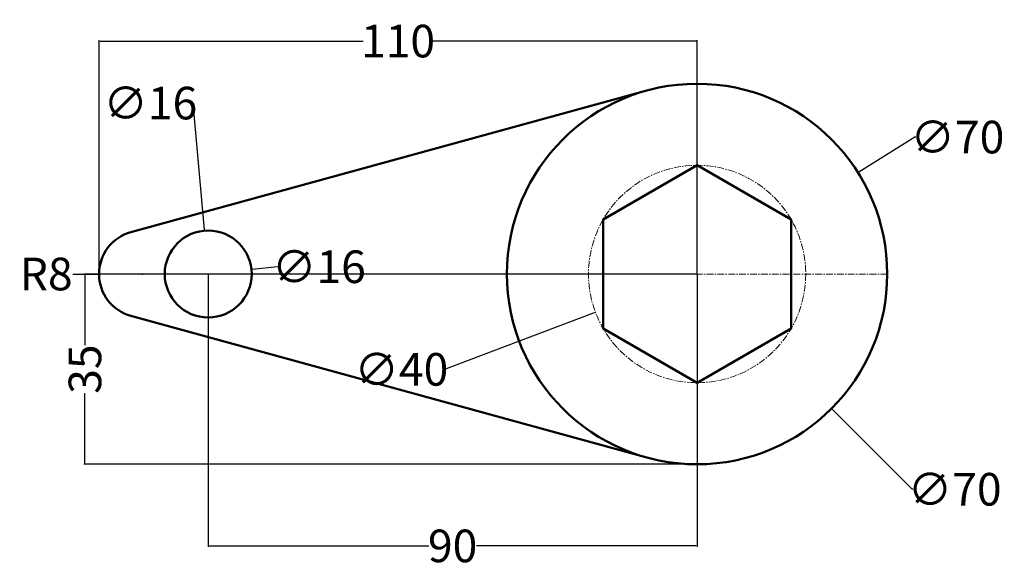
# Model space of a CAD drawing. Units: millimetres. Extents: x -12 to 169, y 16 to 116.
import ezdxf

# ---------------------------------------------------------------- set-up
doc = ezdxf.new("R2010")
doc.units = ezdxf.units.MM
doc.header["$MEASUREMENT"] = 0
doc.linetypes.add('CENTER', pattern=[2, 1.25, -0.25, 0.25, -0.25])
for name, color, linetype, lineweight in [('M-CNTR', 4, 'CENTER', 18), ('M-DIMS', 2, 'Continuous', 25), ('M-OUTL', 7, 'Continuous', 50)]:
    doc.layers.add(name, color=color, linetype=linetype, lineweight=lineweight)
doc.styles.get("Standard").update_dxf_attribs({"font": 'arial.ttf'})
doc.dimstyles.get("Standard").update_dxf_attribs({"dimtxt": 6, "dimasz": 0.18, "dimexe": 0.18, "dimexo": 0.0625, "dimgap": 0.09, "dimtad": 0, "dimtoh": 1, "dimdec": 0, "dimzin": 0, "dimdsep": 46, "dimtxsty": 'Standard', "dimcen": 0.09, "dimadec": 0, "dimazin": 0, "dimtfac": 1, "dimtdec": 0, "dimtofl": 0, "dimtmove": 0, "dimatfit": 3, "dimfxl": 1, "dimtolj": 1, "dimtzin": 0, "dimarcsym": 0})

# ---------------------------------------------------------------- blocks, each defined once
blk = doc.blocks.new('*D1')
at = {"layer": 'Defpoints', "color": 0, "transparency": 16777216}
for p in [(22.94, 69.55), (112.94, 69.55), (112.94, 19.53)]:
    blk.add_point(p, dxfattribs=at)
at = {"layer": 'M-DIMS', "color": 0, "lineweight": -2, "transparency": 16777216}
for p, q in [((22.94, 69.49), (22.94, 19.35)), ((112.94, 69.49), (112.94, 19.35)), ((23.12, 19.53), (63.56, 19.53)), ((112.76, 19.53), (72.31, 19.53))]:
    blk.add_line(p, q, dxfattribs=at)
at = {"layer": 'M-DIMS', "color": 0, "transparency": 16777216}
for points in [[(23.12, 19.56), (23.12, 19.5), (22.94, 19.53)], [(112.76, 19.56), (112.76, 19.5), (112.94, 19.53)]]:
    blk.add_solid(points, dxfattribs=at)
at = {"layer": 'M-DIMS', "color": 0, "transparency": 16777216, "insert": (67.94, 19.53), "char_height": 6, "attachment_point": 5}
blk.add_mtext('\\A1;90', dxfattribs=at)
blk = doc.blocks.new('*D2')
at = {"layer": 'Defpoints', "color": 0, "transparency": 16777216}
for p in [(112.94, 112.4), (2.84, 69.55), (112.94, 69.55)]:
    blk.add_point(p, dxfattribs=at)
at = {"layer": 'M-DIMS', "color": 0, "lineweight": -2, "transparency": 16777216}
for p, q in [((2.84, 69.61), (2.84, 112.58)), ((3.02, 112.4), (51.46, 112.4)), ((112.76, 112.4), (64.31, 112.4)), ((112.94, 69.61), (112.94, 112.58))]:
    blk.add_line(p, q, dxfattribs=at)
at = {"layer": 'M-DIMS', "color": 0, "transparency": 16777216}
for points in [[(3.02, 112.43), (3.02, 112.37), (2.84, 112.4)], [(112.76, 112.43), (112.76, 112.37), (112.94, 112.4)]]:
    blk.add_solid(points, dxfattribs=at)
at = {"layer": 'M-DIMS', "color": 0, "transparency": 16777216, "insert": (57.89, 112.4), "char_height": 6, "attachment_point": 5}
blk.add_mtext('\\A1;110', dxfattribs=at)
blk = doc.blocks.new('*D3')
at = {"layer": 'Defpoints', "color": 0, "transparency": 16777216}
for p in [(22.22, 77.52), (23.65, 61.58)]:
    blk.add_point(p, dxfattribs=at)
at = {"layer": 'M-DIMS', "color": 0, "lineweight": -2, "transparency": 16777216}
for p, q in [((19.92, 101), (20.1, 101)), ((20.1, 101), (22.2, 77.7)), ((22.85, 69.55), (23.03, 69.55)), ((22.94, 69.46), (22.94, 69.64))]:
    blk.add_line(p, q, dxfattribs=at)
at = {"layer": 'M-DIMS', "color": 0, "transparency": 16777216}
blk.add_solid([(22.23, 77.7), (22.17, 77.69), (22.22, 77.52)], dxfattribs=at)
at = {"layer": 'M-DIMS', "color": 0, "transparency": 16777216, "insert": (12.28, 101), "char_height": 6, "attachment_point": 5}
blk.add_mtext('\\A1;∅16', dxfattribs=at)
blk = doc.blocks.new('*D4')
at = {"layer": 'Defpoints', "color": 0, "transparency": 16777216}
for p in [(142.58, 88.17), (83.3, 50.93)]:
    blk.add_point(p, dxfattribs=at)
at = {"layer": 'M-DIMS', "color": 0, "lineweight": -2, "transparency": 16777216}
for p, q in [((153.04, 94.74), (142.73, 88.26)), ((153.22, 94.74), (153.04, 94.74)), ((112.85, 69.55), (113.03, 69.55)), ((112.94, 69.46), (112.94, 69.64))]:
    blk.add_line(p, q, dxfattribs=at)
at = {"layer": 'M-DIMS', "color": 0, "transparency": 16777216}
blk.add_solid([(142.71, 88.29), (142.74, 88.24), (142.58, 88.17)], dxfattribs=at)
at = {"layer": 'M-DIMS', "color": 0, "transparency": 16777216, "insert": (160.86, 94.74), "char_height": 6, "attachment_point": 5}
blk.add_mtext('\\A1;∅70', dxfattribs=at)
blk = doc.blocks.new('*D5')
at = {"layer": 'Defpoints', "color": 0, "transparency": 16777216}
for p in [(131.66, 76.59), (94.22, 62.5)]:
    blk.add_point(p, dxfattribs=at)
at = {"layer": 'M-DIMS', "color": 0, "lineweight": -2, "transparency": 16777216}
for p, q in [((112.85, 69.55), (113.03, 69.55)), ((112.94, 69.46), (112.94, 69.64)), ((66.32, 52.01), (94.05, 62.44)), ((66.14, 52.01), (66.32, 52.01))]:
    blk.add_line(p, q, dxfattribs=at)
at = {"layer": 'M-DIMS', "color": 0, "transparency": 16777216}
blk.add_solid([(94.04, 62.47), (94.06, 62.41), (94.22, 62.5)], dxfattribs=at)
at = {"layer": 'M-DIMS', "color": 0, "transparency": 16777216, "insert": (58.5, 52.01), "char_height": 6, "attachment_point": 5}
blk.add_mtext('\\A1;∅40', dxfattribs=at)
blk = doc.blocks.new('*D6')
at = {"layer": 'Defpoints', "color": 0, "transparency": 16777216}
for p in [(112.85, 69.55), (0.25, 34.55), (112.94, 34.55)]:
    blk.add_point(p, dxfattribs=at)
at = {"layer": 'M-DIMS', "color": 0, "lineweight": -2, "transparency": 16777216}
for p, q in [((112.78, 69.55), (0.07, 69.55)), ((0.25, 69.37), (0.25, 56.46)), ((0.25, 34.73), (0.25, 47.64)), ((112.87, 34.55), (0.07, 34.55))]:
    blk.add_line(p, q, dxfattribs=at)
at = {"layer": 'M-DIMS', "color": 0, "transparency": 16777216}
for points in [[(0.22, 69.37), (0.28, 69.37), (0.25, 69.55)], [(0.22, 34.73), (0.28, 34.73), (0.25, 34.55)]]:
    blk.add_solid(points, dxfattribs=at)
at = {"layer": 'M-DIMS', "color": 0, "transparency": 16777216, "insert": (0.25, 52.05), "char_height": 6, "attachment_point": 5, "rotation": 90}
blk.add_mtext('\\A1;35', dxfattribs=at)
blk = doc.blocks.new('*D7')
at = {"layer": 'Defpoints', "color": 0, "transparency": 16777216}
for p in [(88.19, 94.3), (137.69, 44.8)]:
    blk.add_point(p, dxfattribs=at)
at = {"layer": 'M-DIMS', "color": 0, "lineweight": -2, "transparency": 16777216}
for p, q in [((112.85, 69.55), (113.03, 69.55)), ((112.94, 69.46), (112.94, 69.64)), ((152.53, 29.95), (137.81, 44.67)), ((152.71, 29.95), (152.53, 29.95))]:
    blk.add_line(p, q, dxfattribs=at)
at = {"layer": 'M-DIMS', "color": 0, "transparency": 16777216}
blk.add_solid([(137.83, 44.69), (137.79, 44.65), (137.69, 44.8)], dxfattribs=at)
at = {"layer": 'M-DIMS', "color": 0, "transparency": 16777216, "insert": (160.36, 29.95), "char_height": 6, "attachment_point": 5}
blk.add_mtext('\\A1;∅70', dxfattribs=at)
blk = doc.blocks.new('*D8')
at = {"layer": 'Defpoints', "color": 0, "transparency": 16777216}
for p in [(2.84, 69.55), (10.84, 69.55)]:
    blk.add_point(p, dxfattribs=at)
at = {"layer": 'M-DIMS', "color": 0, "lineweight": -2, "transparency": 16777216}
for p, q in [((-1.96, 69.55), (2.66, 69.55)), ((10.75, 69.55), (10.93, 69.55)), ((10.84, 69.46), (10.84, 69.64))]:
    blk.add_line(p, q, dxfattribs=at)
at = {"layer": 'M-DIMS', "color": 0, "transparency": 16777216}
blk.add_solid([(2.66, 69.58), (2.66, 69.52), (2.84, 69.55)], dxfattribs=at)
at = {"layer": 'M-DIMS', "color": 0, "transparency": 16777216, "insert": (-6.89, 69.55), "char_height": 6, "attachment_point": 5}
blk.add_mtext('\\A1;R8', dxfattribs=at)
blk = doc.blocks.new('*D9')
at = {"layer": 'Defpoints', "color": 0, "transparency": 16777216}
for p in [(30.89, 70.39), (14.98, 68.71)]:
    blk.add_point(p, dxfattribs=at)
at = {"layer": 'M-DIMS', "color": 0, "lineweight": -2, "transparency": 16777216}
for p, q in [((35.67, 70.89), (31.07, 70.4)), ((22.85, 69.55), (23.03, 69.55)), ((22.94, 69.46), (22.94, 69.64))]:
    blk.add_line(p, q, dxfattribs=at)
at = {"layer": 'M-DIMS', "color": 0, "transparency": 16777216}
blk.add_solid([(31.07, 70.43), (31.08, 70.37), (30.89, 70.39)], dxfattribs=at)
at = {"layer": 'M-DIMS', "color": 0, "transparency": 16777216, "insert": (43.32, 70.89), "char_height": 6, "attachment_point": 5}
blk.add_mtext('\\A1;∅16', dxfattribs=at)

msp = doc.modelspace()

# ---------------------------------------------------------------- linework, layer by layer
at = {"layer": 'M-CNTR'}
msp.add_lwpolyline([(147.94, 69.55), (14.94, 69.55), (2.94, 69.55)], dxfattribs=at)
msp.add_circle((112.94, 69.55), 20, dxfattribs=at)
at = {"layer": 'M-OUTL'}
msp.add_lwpolyline([(103.68, 35.79), (8.72, 61.83, -0.762701), (8.72, 77.26), (103.68, 103.3)], format="xyb", dxfattribs=at)
msp.add_lwpolyline([(112.94, 49.55), (130.26, 59.55), (130.26, 79.55), (112.94, 89.55), (95.62, 79.55), (95.62, 59.55)], close=True, dxfattribs=at)
for centre, radius in [((112.94, 69.55), 35), ((22.94, 69.55), 8)]:
    msp.add_circle(centre, radius, dxfattribs=at)

# ---------------------------------------------------------------- dimensions: what is measured, and where the dimension line sits
at = {"layer": 'M-DIMS'}
for base, p1, picture, middle in [((112.94, 112.4), (2.84, 69.55), '*D2', (57.89, 112.4)), ((112.94, 19.53), (22.94, 69.55), '*D1', (67.94, 19.53))]:
    dim = msp.add_linear_dim(base=base, p1=p1, p2=(112.94, 69.55), dimstyle='Standard', override={"dimclrd": 0, "dimclre": 0, "dimclrt": 0}, dxfattribs=at)
    dim.commit()
    dim.dimension.update_dxf_attribs({"geometry": picture, "text_midpoint": middle})
for p1, p2, override, picture, middle in [((23.65, 61.58), (22.22, 77.52), {"dimclrd": 0, "dimclre": 0, "dimclrt": 0}, '*D3', (12.28, 101)), ((83.3, 50.93), (142.58, 88.17), {"dimclrd": 0, "dimclre": 0, "dimclrt": 0}, '*D4', (160.86, 94.74)), ((88.19, 94.3), (137.69, 44.8), {"dimdec": 0, "dimlfac": 1, "dimrnd": 0, "dimzin": 0, "dimdsep": 46, "dimlunit": 2}, '*D7', (160.36, 29.95)), ((131.66, 76.59), (94.22, 62.5), {"dimclrd": 0, "dimclre": 0, "dimclrt": 0}, '*D5', (58.5, 52.01)), ((14.98, 68.71), (30.89, 70.39), {"dimdec": 0, "dimlfac": 1, "dimrnd": 0, "dimzin": 0, "dimdsep": 46, "dimlunit": 2}, '*D9', (35.67, 70.89))]:
    dim = msp.add_diameter_dim_2p(p1=p1, p2=p2, dimstyle='Standard', override=override, dxfattribs=at)
    dim.commit()
    dim.dimension.update_dxf_attribs({"geometry": picture, "text_midpoint": middle, "dimtype": 163})
dim = msp.add_radius_dim(center=(10.84, 69.55), mpoint=(2.84, 69.55), dimstyle='Standard', override={"dimdec": 0, "dimlfac": 1, "dimrnd": 0, "dimzin": 0, "dimdsep": 46, "dimlunit": 2}, dxfattribs=at)
dim.commit()
dim.dimension.update_dxf_attribs({"geometry": '*D8', "text_midpoint": (-1.96, 69.55), "dimtype": 164})
dim = msp.add_linear_dim(base=(0.25, 34.55), p1=(112.85, 69.55), p2=(112.94, 34.55), angle=90, dimstyle='Standard', override={"dimclrd": 0, "dimclre": 0, "dimclrt": 0}, dxfattribs=at)
dim.commit()
dim.dimension.update_dxf_attribs({"geometry": '*D6', "text_midpoint": (0.25, 52.05)})

doc.saveas('drawing.dxf')
